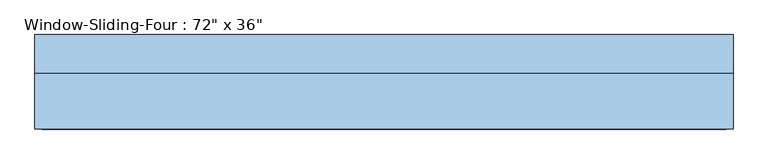
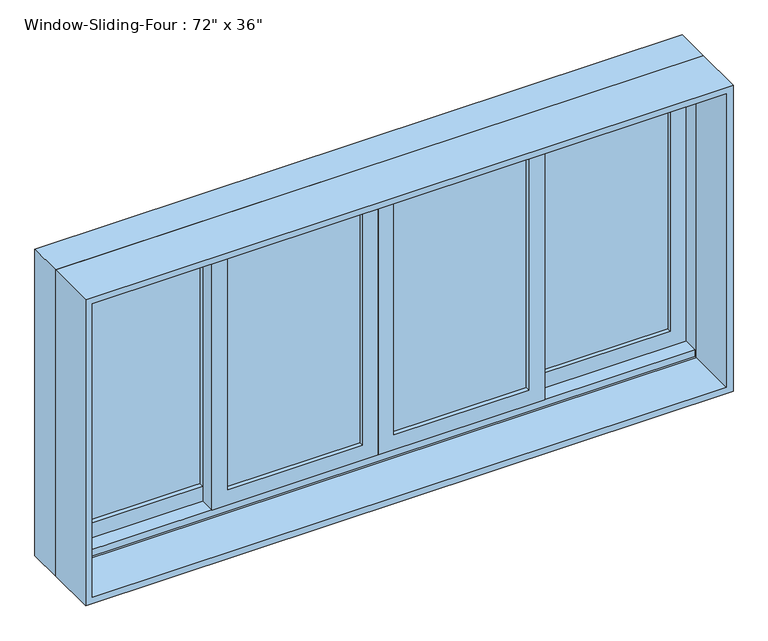
"""IFC4 building model written with IfcOpenShell, lengths in millimetres: window geometry."""

from ifc_helpers import new_model, si_unit, frame, origin, place, context, project, spatial, polyline, outline, extrude, faceted_brep, source, transform, mapped, element, save


def window_58cce754(model_context):
    return source(origin(), model_context, "Body", "SolidModel", [
        extrude(outline(polyline([(933.45, -895.35), (933.45, -425.45), (1809.75, -425.45), (1809.75, -895.35), (933.45, -895.35)]), holes=[polyline([(1765.3, -469.9), (996.95, -469.9), (996.95, -850.9), (1765.3, -850.9), (1765.3, -469.9)])]), frame((0.0, 78.74, 0.0), z_axis=(0.0, 1.0, 0.0), x_axis=(0.0, 0.0, 1.0)), (0.0, 0.0, 1.0), 44.45),
        extrude(outline(polyline([(-469.9, 110.49), (-469.9, 104.14), (-850.9, 104.14), (-850.9, 110.49), (-469.9, 110.49)])), frame((0.0, 0.0, 996.95), z_axis=(0.0, 0.0, 1.0), x_axis=(1.0, 0.0, 0.0)), (0.0, 0.0, 1.0), 768.35),
        extrude(outline(polyline([(-469.9, 97.79), (-469.9, 91.44), (-850.9, 91.44), (-850.9, 97.79), (-469.9, 97.79)])), frame((0.0, 0.0, 996.95), z_axis=(0.0, 0.0, 1.0), x_axis=(1.0, 0.0, 0.0)), (0.0, 0.0, 1.0), 768.35),
        extrude(outline(polyline([(-44.45, 66.04), (-44.45, 59.69), (-425.45, 59.69), (-425.45, 66.04), (-44.45, 66.04)])), frame((0.0, 0.0, 996.95), z_axis=(0.0, 0.0, 1.0), x_axis=(1.0, 0.0, 0.0)), (0.0, 0.0, 1.0), 768.35),
        extrude(outline(polyline([(-44.45, 53.34), (-44.45, 46.99), (-425.45, 46.99), (-425.45, 53.34), (-44.45, 53.34)])), frame((0.0, 0.0, 996.95), z_axis=(0.0, 0.0, 1.0), x_axis=(1.0, 0.0, 0.0)), (0.0, 0.0, 1.0), 768.35),
        extrude(outline(polyline([(1828.8, -914.4), (914.4, -914.4), (914.4, 914.4), (1828.8, 914.4), (1828.8, -914.4)]), holes=[polyline([(1809.75, 895.35), (933.45, 895.35), (933.45, -895.35), (1809.75, -895.35), (1809.75, 895.35)])]), frame((0.0, -118.11, 0.0), z_axis=(0.0, 1.0, 0.0), x_axis=(0.0, 0.0, 1.0)), (0.0, 0.0, 1.0), 146.05),
        extrude(outline(polyline([(952.5, 469.9), (1809.75, 469.9), (1809.75, 0.0), (952.5, 0.0), (952.5, 469.9)]), holes=[polyline([(996.95, 44.45), (1765.3, 44.45), (1765.3, 425.45), (996.95, 425.45), (996.95, 44.45)])]), frame((0.0, 34.29, 0.0), z_axis=(0.0, 1.0, 0.0), x_axis=(0.0, 0.0, 1.0)), (0.0, 0.0, 1.0), 44.45),
        extrude(outline(polyline([(1809.75, -469.9), (952.5, -469.9), (952.5, 0.0), (1809.75, 0.0), (1809.75, -469.9)]), holes=[polyline([(1765.3, -44.45), (996.95, -44.45), (996.95, -425.45), (1765.3, -425.45), (1765.3, -44.45)])]), frame((0.0, 34.29, 0.0), z_axis=(0.0, 1.0, 0.0), x_axis=(0.0, 0.0, 1.0)), (0.0, 0.0, 1.0), 44.45),
        extrude(outline(polyline([(425.45, 66.04), (425.45, 59.69), (44.45, 59.69), (44.45, 66.04), (425.45, 66.04)])), frame((0.0, 0.0, 996.95), z_axis=(0.0, 0.0, 1.0), x_axis=(1.0, 0.0, 0.0)), (0.0, 0.0, 1.0), 768.35),
        extrude(outline(polyline([(425.45, 53.34), (425.45, 46.99), (44.45, 46.99), (44.45, 53.34), (425.45, 53.34)])), frame((0.0, 0.0, 996.95), z_axis=(0.0, 0.0, 1.0), x_axis=(1.0, 0.0, 0.0)), (0.0, 0.0, 1.0), 768.35),
        extrude(outline(polyline([(850.9, 110.49), (850.9, 104.14), (469.9, 104.14), (469.9, 110.49), (850.9, 110.49)])), frame((0.0, 0.0, 996.95), z_axis=(0.0, 0.0, 1.0), x_axis=(1.0, 0.0, 0.0)), (0.0, 0.0, 1.0), 768.35),
        extrude(outline(polyline([(850.9, 97.4725303), (850.9, 91.44), (469.9, 91.44), (469.9, 97.4725303), (850.9, 97.4725303)])), frame((0.0, 0.0, 996.95), z_axis=(0.0, 0.0, 1.0), x_axis=(1.0, 0.0, 0.0)), (0.0, 0.0, 1.0), 768.35),
        extrude(outline(polyline([(933.45, 895.35), (1809.75, 895.35), (1809.75, 425.45), (933.45, 425.45), (933.45, 895.35)]), holes=[polyline([(1765.3, 469.9), (1765.3, 850.9), (996.95, 850.9), (996.95, 469.9), (1765.3, 469.9)])]), frame((0.0, 78.74, 0.0), z_axis=(0.0, 1.0, 0.0), x_axis=(0.0, 0.0, 1.0)), (0.0, 0.0, 1.0), 44.45),
        faceted_brep([(-914.4, 27.94, 914.4), (-914.4, 129.54, 914.4), (914.4, 129.54, 914.4), (914.4, 27.94, 914.4), (-873.4778905, 129.54, 1787.8778905), (-873.4778905, 123.19, 1787.8778905), (-873.4778905, 123.19, 933.45), (-873.4778905, 129.54, 933.45), (873.4778905, 123.19, 1787.8778905), (873.4778905, 123.19, 933.45), (895.35, 123.19, 933.45), (895.35, 123.19, 1809.75), (-895.35, 123.19, 1809.75), (-895.35, 123.19, 933.45), (-895.35, 27.94, 1809.75), (-895.35, 27.94, 933.45), (-895.35, 34.29, 933.45), (-895.35, 34.29, 952.5), (-895.35, 78.74, 952.5), (-895.35, 78.74, 933.45), (914.4, 27.94, 1828.8), (-914.4, 27.94, 1828.8), (895.35, 27.94, 1809.75), (895.35, 27.94, 933.45), (-914.4, 129.54, 1828.8), (914.4, 129.54, 1828.8), (873.4778905, 129.54, 933.45), (873.4778905, 129.54, 1787.8778905), (895.35, 78.74, 933.45), (895.35, 78.74, 952.5), (895.35, 34.29, 952.5), (895.35, 34.29, 933.45)], [[[0, 1, 2, 3]], [[4, 5, 6, 7]], [[5, 8, 9, 10, 11, 12, 13, 6]], [[12, 14, 15, 16, 17, 18, 19, 13]], [[0, 3, 20, 21], [22, 23, 15, 14]], [[24, 1, 0, 21]], [[2, 1, 24, 25], [4, 7, 26, 27]], [[5, 4, 27, 8]], [[12, 11, 22, 14]], [[21, 20, 25, 24]], [[8, 27, 26, 9]], [[22, 11, 10, 28, 29, 30, 31, 23]], [[20, 3, 2, 25]], [[26, 7, 6, 13, 19, 28, 10, 9]], [[28, 19, 18, 29]], [[29, 18, 17, 30]], [[30, 17, 16, 31]], [[15, 23, 31, 16]]]),
    ])


if __name__ == "__main__":
    model = new_model("IFC4")
    model_context = context("Model", 3, world=origin())
    ifc_project = project(units=[si_unit("LENGTHUNIT", "METRE", prefix="MILLI")], contexts=[model_context])
    site = spatial("IfcSite", under=ifc_project)
    building = spatial("IfcBuilding", under=site)
    placement = place(None, origin())
    window_shape = window_58cce754(model_context)
    element("IfcWindow", 1, ObjectType="Window-Sliding-Four : 72\" x 36\"", at=placement, inside=building, context=model_context, shape_type="MappedRepresentation", body=[
        mapped(window_shape, transform((0.0, 0.0, 0.0), x_axis=(1.0, 0.0, 0.0), y_axis=(0.0, 1.0, 0.0), z_axis=(0.0, 0.0, 1.0))),
    ])
    save(model, "model.ifc")

# Revit data of these elements
# Type "Window-Sliding-Four : 72\" x 36\""
#   Type Mark = "20"
#   Fire Rating = "0.5h"
#   Assembly Code = "B2020100"
#   Analytic Construction = "Double glazing - domestic"
#   Window Inset [instance default] = 0' - 0"
#   Wall Thickness [instance default] = 0' - 6"
#   Visual Light Transmittance = 0.81
#   Thermal Resistance (R) = 1.8146 (h·ft²·°F)/BTU
#   Solar Heat Gain Coefficient = 0.76
#   Interior Wall Closure [instance default] = 0' - 2 19/32"
#   Heat Transfer Coefficient (U) = 0.5511 BTU/(h·ft²·°F)
#   Frame Extension [instance default] = 0' - 0 1/4"
#   Exterior Wall Closure [instance default] = 0' - 1 1/4"
#   Rough Width = 6' - 0 1/2"
#   Rough Height = 3' - 0 1/2"
#   Height = 3' - 0"
#   Extension Jamb [instance default] = 0' - 2 3/4"
#   Default Sill Height = 3' - 0"
#   Width = 6' - 0"
#   Middle Muntin Visibility = yes
#   Interior Trim Visibility [instance default] = yes
#   Indicator Visibility [instance default] = yes
#   Exterior Trim Visibility [instance default] = yes
#   Side Muntin Visibility = yes
#   Extension Jamb Visibility [instance default] = yes
#   Interior Trim Material = Wood - Stained
#   Muntin Pattern = Muntin Pattern_2x2 : Muntin Pattern_2x2
#   Interior Trim = Trim-Window-Interior-Flat : Picture Frame
#   Interior Frame Material = Wood - Stained
#   Glass Panel Material = Glass
#   Exterior Trim Material = Clad - White
#   Exterior Trim = Trim-Window-Exterior-Flat : with Sill
#   Exterior Frame Material = Clad - White
#   Wall Closure = (empty or 0)
# Element 1 (IfcWindow, "Window-Sliding-Four : 72\" x 36\"")
#   Wall Thickness = 0' - 9"
#   Extension Jamb = 0' - 5 3/4"
#   Materials on its faces: "Wood - Stained", "Glass", "Clad - White"
# Materials
#   "Wood - Stained": class "Wood", colour RGB 224 178 126, transparency 0, Cost = 0
#   "Glass": class "Glass", colour RGB 0 128 192, transparency 0.75, Description = "Soda Lime Glass", Cost = 0
#   "Clad - White": class "Wood", colour RGB 242 242 238, transparency 0, Cost = 0
